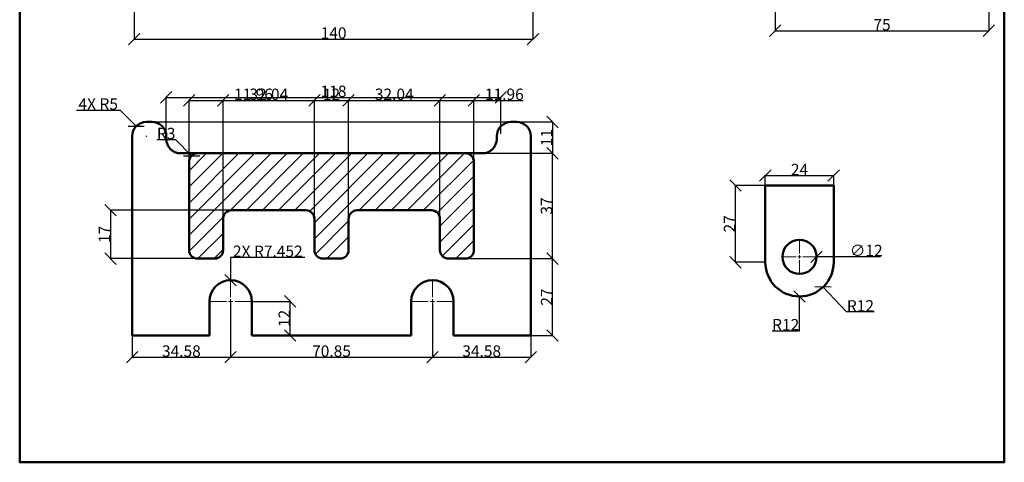
# Model space of a CAD drawing. Units: millimetres. Extents: x -13 to 343, y 323 to 787.
# Tile 1 of 3: x -13 to 333, y 323 to 479. Entities that reach past the tile are written whole.
import ezdxf

# ---------------------------------------------------------------- set-up
doc = ezdxf.new("R2010")
doc.units = ezdxf.units.MM
doc.header["$MEASUREMENT"] = 0
doc.header["$PDMODE"] = 3
doc.header["$PDSIZE"] = -8
doc.linetypes.add('CENTER', pattern=[50.8, 31.75, -6.35, 6.35, -6.35])
for name, color, linetype, lineweight in [('M-CNTR', 1, 'CENTER', 18), ('M-DIMS', 2, 'Continuous', 25), ('M-HATC', 8, 'Continuous', 18), ('M-OUTL', 7, 'Continuous', 50), ('M-TTLB', 7, 'Continuous', 50)]:
    doc.layers.add(name, color=color, linetype=linetype, lineweight=lineweight)
doc.styles.get("Standard").update_dxf_attribs({"font": 'arial.ttf'})
doc.dimstyles.get("Standard").update_dxf_attribs({"dimtxt": 4, "dimasz": 4, "dimexe": 0.18, "dimexo": 0.0625, "dimgap": 0.09, "dimtad": 1, "dimtoh": 1, "dimdec": 0, "dimzin": 0, "dimdsep": 46, "dimtxsty": 'Standard', "dimblk": 'OBLIQUE', "dimcen": 0.09, "dimclre": 251, "dimadec": 0, "dimazin": 0, "dimtfac": 1, "dimtdec": 0, "dimtofl": 0, "dimtmove": 0, "dimatfit": 3, "dimfxl": 1, "dimtolj": 1, "dimtzin": 0, "dimarcsym": 0})

# ---------------------------------------------------------------- blocks, each defined once
blk = doc.blocks.new('*U2')
at = {"layer": 'M-CNTR', "color": 0, "transparency": 16777216}
for p, q in [((0, 1.49), (0, 7.57)), ((-7.57, 0), (-1.49, 0)), ((1.49, 0), (7.57, 0)), ((0, -7.57), (0, -1.49))]:
    blk.add_line(p, q, dxfattribs=at)
at = {"layer": 'M-CNTR', "color": 0, "linetype": 'Continuous', "transparency": 16777216}
for p, q in [((-0.75, 0), (0.75, 0)), ((0, -0.75), (0, 0.75))]:
    blk.add_line(p, q, dxfattribs=at)
blk = doc.blocks.new('*U3')
at = {"layer": 'M-CNTR', "color": 0, "transparency": 16777216}
for p, q in [((0, 1.49), (0, 7.57)), ((-7.57, 0), (-1.49, 0)), ((1.49, 0), (7.57, 0)), ((0, -7.57), (0, -1.49))]:
    blk.add_line(p, q, dxfattribs=at)
at = {"layer": 'M-CNTR', "color": 0, "linetype": 'Continuous', "transparency": 16777216}
for p, q in [((-0.75, 0), (0.75, 0)), ((0, -0.75), (0, 0.75))]:
    blk.add_line(p, q, dxfattribs=at)
blk = doc.blocks.new('_Oblique')
at = {"color": 0, "linetype": 'ByBlock', "lineweight": -2}
blk.add_line((-0.5, -0.5), (0.5, 0.5), dxfattribs=at)
blk = doc.blocks.new('*D15')
at = {"layer": 'Defpoints', "color": 0, "transparency": 16777216}
for p in [(27.05, 495.9), (167.05, 495.9), (167.05, 471.86)]:
    blk.add_point(p, dxfattribs=at)
at = {"layer": 'M-DIMS', "color": 0, "lineweight": -2, "transparency": 16777216}
for p, q in [((27.05, 495.83), (27.05, 471.68)), ((167.05, 495.83), (167.05, 471.68)), ((27.05, 471.86), (167.05, 471.86))]:
    blk.add_line(p, q, dxfattribs=at)
at = {"layer": 'M-DIMS', "color": 0, "lineweight": -2, "transparency": 16777216, "xscale": 4, "yscale": 4, "zscale": 4, "rotation": 180}
blk.add_blockref('_Oblique', (27.05, 471.86), dxfattribs=at)
at = {"layer": 'M-DIMS', "color": 0, "lineweight": -2, "transparency": 16777216, "xscale": 4, "yscale": 4, "zscale": 4}
blk.add_blockref('_Oblique', (167.05, 471.86), dxfattribs=at)
at = {"layer": 'M-DIMS', "color": 0, "transparency": 16777216, "insert": (97.05, 473.99), "char_height": 4, "attachment_point": 5}
blk.add_mtext('\\A1;140', dxfattribs=at)
blk = doc.blocks.new('*D32')
at = {"layer": 'Defpoints', "color": 0, "transparency": 16777216}
for p in [(252.08, 495.9), (327.08, 495.9), (327.08, 474.82)]:
    blk.add_point(p, dxfattribs=at)
at = {"layer": 'M-DIMS', "color": 0, "lineweight": -2, "transparency": 16777216}
for p, q in [((252.08, 495.83), (252.08, 474.64)), ((327.08, 495.83), (327.08, 474.64)), ((252.08, 474.82), (327.08, 474.82))]:
    blk.add_line(p, q, dxfattribs=at)
at = {"layer": 'M-DIMS', "color": 0, "lineweight": -2, "transparency": 16777216, "xscale": 4, "yscale": 4, "zscale": 4, "rotation": 180}
blk.add_blockref('_Oblique', (252.08, 474.82), dxfattribs=at)
at = {"layer": 'M-DIMS', "color": 0, "lineweight": -2, "transparency": 16777216, "xscale": 4, "yscale": 4, "zscale": 4}
blk.add_blockref('_Oblique', (327.08, 474.82), dxfattribs=at)
at = {"layer": 'M-DIMS', "color": 0, "transparency": 16777216, "insert": (289.58, 476.94), "char_height": 4, "attachment_point": 5}
blk.add_mtext('\\A1;75', dxfattribs=at)
blk = doc.blocks.new('*D33')
at = {"layer": 'Defpoints', "color": 0, "transparency": 16777216}
for p in [(155.79, 451.41), (38.28, 438.48), (155.79, 438.48)]:
    blk.add_point(p, dxfattribs=at)
at = {"layer": 'M-DIMS', "color": 0, "lineweight": -2, "transparency": 16777216}
for p, q in [((38.28, 438.54), (38.28, 451.59)), ((38.28, 451.41), (155.79, 451.41)), ((155.79, 438.54), (155.79, 451.59))]:
    blk.add_line(p, q, dxfattribs=at)
at = {"layer": 'M-DIMS', "color": 0, "lineweight": -2, "transparency": 16777216, "xscale": 4, "yscale": 4, "zscale": 4, "rotation": 180}
blk.add_blockref('_Oblique', (38.28, 451.41), dxfattribs=at)
at = {"layer": 'M-DIMS', "color": 0, "lineweight": -2, "transparency": 16777216, "xscale": 4, "yscale": 4, "zscale": 4}
blk.add_blockref('_Oblique', (155.79, 451.41), dxfattribs=at)
at = {"layer": 'M-DIMS', "color": 0, "transparency": 16777216, "insert": (97.03, 453.54), "char_height": 4, "attachment_point": 5}
blk.add_mtext('\\A1;118', dxfattribs=at)
blk = doc.blocks.new('*D34')
at = {"layer": 'Defpoints', "color": 0, "transparency": 16777216}
for p in [(68.48, 379.75), (81.84, 379.75), (75.74, 367.75)]:
    blk.add_point(p, dxfattribs=at)
at = {"layer": 'M-DIMS', "color": 0, "lineweight": -2, "transparency": 16777216}
for p, q in [((68.54, 379.75), (82.02, 379.75)), ((81.84, 367.75), (81.84, 379.75)), ((75.8, 367.75), (82.02, 367.75))]:
    blk.add_line(p, q, dxfattribs=at)
at = {"layer": 'M-DIMS', "color": 0, "lineweight": -2, "transparency": 16777216, "xscale": 4, "yscale": 4, "zscale": 4}
for p, rotation in [((81.84, 379.75), 90), ((81.84, 367.75), 270)]:
    blk.add_blockref('_Oblique', p, dxfattribs=dict(at, rotation=rotation))
at = {"layer": 'M-DIMS', "color": 0, "transparency": 16777216, "insert": (79.74, 373.75), "char_height": 4, "attachment_point": 5, "rotation": 90}
blk.add_mtext('\\A1;12', dxfattribs=at)
blk = doc.blocks.new('*U35')
at = {"layer": 'M-CNTR', "color": 0, "transparency": 16777216}
for p, q in [((0, 1.2), (0, 6.12)), ((-6.12, 0), (-1.2, 0)), ((1.2, 0), (6.12, 0)), ((0, -6.12), (0, -1.2))]:
    blk.add_line(p, q, dxfattribs=at)
at = {"layer": 'M-CNTR', "color": 0, "linetype": 'Continuous', "transparency": 16777216}
for p, q in [((-0.6, 0), (0.6, 0)), ((0, -0.6), (0, 0.6))]:
    blk.add_line(p, q, dxfattribs=at)
blk = doc.blocks.new('*D36')
at = {"layer": 'Defpoints', "color": 0, "transparency": 16777216}
for p in [(238.13, 420.46), (248.61, 420.46), (248.61, 393.46)]:
    blk.add_point(p, dxfattribs=at)
at = {"layer": 'M-DIMS', "color": 0, "lineweight": -2, "transparency": 16777216}
for p, q in [((248.54, 420.46), (237.95, 420.46)), ((238.13, 393.46), (238.13, 420.46)), ((248.54, 393.46), (237.95, 393.46))]:
    blk.add_line(p, q, dxfattribs=at)
at = {"layer": 'M-DIMS', "color": 0, "lineweight": -2, "transparency": 16777216, "xscale": 4, "yscale": 4, "zscale": 4}
for p, rotation in [((238.13, 420.46), 90), ((238.13, 393.46), 270)]:
    blk.add_blockref('_Oblique', p, dxfattribs=dict(at, rotation=rotation))
at = {"layer": 'M-DIMS', "color": 0, "transparency": 16777216, "insert": (236.03, 406.96), "char_height": 4, "attachment_point": 5, "rotation": 90}
blk.add_mtext('\\A1;27', dxfattribs=at)
blk = doc.blocks.new('*D37')
at = {"layer": 'Defpoints', "color": 0, "transparency": 16777216}
for p in [(260.61, 393.46), (268.87, 384.77)]:
    blk.add_point(p, dxfattribs=at)
at = {"layer": 'M-DIMS', "color": 0, "lineweight": -2, "transparency": 16777216}
for p, q in [((260.52, 393.46), (260.7, 393.46)), ((260.61, 393.37), (260.61, 393.55)), ((277.15, 376.06), (268.87, 384.77)), ((286.76, 376.06), (277.15, 376.06))]:
    blk.add_line(p, q, dxfattribs=at)
at = {"layer": 'M-DIMS', "color": 0, "lineweight": -2, "transparency": 16777216, "xscale": 4, "yscale": 4, "zscale": 4, "rotation": 133.5491002898065}
blk.add_blockref('_Oblique', (268.87, 384.77), dxfattribs=at)
at = {"layer": 'M-DIMS', "color": 0, "transparency": 16777216, "insert": (282, 378.16), "char_height": 4, "attachment_point": 5}
blk.add_mtext('\\A1;R12', dxfattribs=at)
blk = doc.blocks.new('*D45')
at = {"layer": 'Defpoints', "color": 0, "transparency": 16777216}
for p in [(60.91, 379.75), (26.33, 367.75), (60.91, 360.15)]:
    blk.add_point(p, dxfattribs=at)
at = {"layer": 'M-DIMS', "color": 251, "lineweight": -2, "transparency": 16777216}
for p, q in [((60.91, 379.69), (60.91, 359.97)), ((26.33, 367.69), (26.33, 359.97))]:
    blk.add_line(p, q, dxfattribs=at)
at = {"layer": 'M-DIMS', "color": 0, "lineweight": -2, "transparency": 16777216}
blk.add_line((26.33, 360.15), (60.91, 360.15), dxfattribs=at)
at = {"layer": 'M-DIMS', "color": 0, "lineweight": -2, "transparency": 16777216, "xscale": 4, "yscale": 4, "zscale": 4, "rotation": 180}
blk.add_blockref('_Oblique', (26.33, 360.15), dxfattribs=at)
at = {"layer": 'M-DIMS', "color": 0, "lineweight": -2, "transparency": 16777216, "xscale": 4, "yscale": 4, "zscale": 4}
blk.add_blockref('_Oblique', (60.91, 360.15), dxfattribs=at)
at = {"layer": 'M-DIMS', "color": 0, "transparency": 16777216, "insert": (43.62, 362.28), "char_height": 4, "attachment_point": 5}
blk.add_mtext('\\A1;34.58', dxfattribs=at)
blk = doc.blocks.new('*D46')
at = {"layer": 'Defpoints', "color": 0, "transparency": 16777216}
for p in [(60.91, 379.75), (131.75, 379.75), (131.75, 360.15)]:
    blk.add_point(p, dxfattribs=at)
at = {"layer": 'M-DIMS', "color": 251, "lineweight": -2, "transparency": 16777216}
for p, q in [((60.91, 379.69), (60.91, 359.97)), ((131.75, 379.69), (131.75, 359.97))]:
    blk.add_line(p, q, dxfattribs=at)
at = {"layer": 'M-DIMS', "color": 0, "lineweight": -2, "transparency": 16777216}
blk.add_line((60.91, 360.15), (131.75, 360.15), dxfattribs=at)
at = {"layer": 'M-DIMS', "color": 0, "lineweight": -2, "transparency": 16777216, "xscale": 4, "yscale": 4, "zscale": 4, "rotation": 180}
blk.add_blockref('_Oblique', (60.91, 360.15), dxfattribs=at)
at = {"layer": 'M-DIMS', "color": 0, "lineweight": -2, "transparency": 16777216, "xscale": 4, "yscale": 4, "zscale": 4}
blk.add_blockref('_Oblique', (131.75, 360.15), dxfattribs=at)
at = {"layer": 'M-DIMS', "color": 0, "transparency": 16777216, "insert": (96.33, 362.28), "char_height": 4, "attachment_point": 5}
blk.add_mtext('\\A1;70.85', dxfattribs=at)
blk = doc.blocks.new('*D47')
at = {"layer": 'Defpoints', "color": 0, "transparency": 16777216}
for p in [(131.75, 379.75), (166.33, 367.75), (166.33, 360.15)]:
    blk.add_point(p, dxfattribs=at)
at = {"layer": 'M-DIMS', "color": 251, "lineweight": -2, "transparency": 16777216}
for p, q in [((131.75, 379.69), (131.75, 359.97)), ((166.33, 367.69), (166.33, 359.97))]:
    blk.add_line(p, q, dxfattribs=at)
at = {"layer": 'M-DIMS', "color": 0, "lineweight": -2, "transparency": 16777216}
blk.add_line((131.75, 360.15), (166.33, 360.15), dxfattribs=at)
at = {"layer": 'M-DIMS', "color": 0, "lineweight": -2, "transparency": 16777216, "xscale": 4, "yscale": 4, "zscale": 4, "rotation": 180}
blk.add_blockref('_Oblique', (131.75, 360.15), dxfattribs=at)
at = {"layer": 'M-DIMS', "color": 0, "lineweight": -2, "transparency": 16777216, "xscale": 4, "yscale": 4, "zscale": 4}
blk.add_blockref('_Oblique', (166.33, 360.15), dxfattribs=at)
at = {"layer": 'M-DIMS', "color": 0, "transparency": 16777216, "insert": (149.04, 362.28), "char_height": 4, "attachment_point": 5}
blk.add_mtext('\\A1;34.58', dxfattribs=at)
blk = doc.blocks.new('*D48')
at = {"layer": 'Defpoints', "color": 0, "transparency": 16777216}
for p in [(33.33, 442.75), (43.33, 431.75), (173.93, 431.75)]:
    blk.add_point(p, dxfattribs=at)
at = {"layer": 'M-DIMS', "color": 251, "lineweight": -2, "transparency": 16777216}
for p, q in [((33.39, 442.75), (174.11, 442.75)), ((43.39, 431.75), (174.11, 431.75))]:
    blk.add_line(p, q, dxfattribs=at)
at = {"layer": 'M-DIMS', "color": 0, "lineweight": -2, "transparency": 16777216}
blk.add_line((173.93, 442.75), (173.93, 431.75), dxfattribs=at)
at = {"layer": 'M-DIMS', "color": 0, "lineweight": -2, "transparency": 16777216, "xscale": 4, "yscale": 4, "zscale": 4}
for p, rotation in [((173.93, 442.75), 90), ((173.93, 431.75), 270)]:
    blk.add_blockref('_Oblique', p, dxfattribs=dict(at, rotation=rotation))
at = {"layer": 'M-DIMS', "color": 0, "transparency": 16777216, "insert": (171.83, 437.25), "char_height": 4, "attachment_point": 5, "rotation": 90}
blk.add_mtext('\\A1;11', dxfattribs=at)
blk = doc.blocks.new('*D49')
at = {"layer": 'Defpoints', "color": 0, "transparency": 16777216}
for p in [(143.33, 394.75), (173.93, 394.75), (166.33, 367.75)]:
    blk.add_point(p, dxfattribs=at)
at = {"layer": 'M-DIMS', "color": 251, "lineweight": -2, "transparency": 16777216}
for p, q in [((143.39, 394.75), (174.11, 394.75)), ((166.39, 367.75), (174.11, 367.75))]:
    blk.add_line(p, q, dxfattribs=at)
at = {"layer": 'M-DIMS', "color": 0, "lineweight": -2, "transparency": 16777216}
blk.add_line((173.93, 367.75), (173.93, 394.75), dxfattribs=at)
at = {"layer": 'M-DIMS', "color": 0, "lineweight": -2, "transparency": 16777216, "xscale": 4, "yscale": 4, "zscale": 4}
for p, rotation in [((173.93, 394.75), 90), ((173.93, 367.75), 270)]:
    blk.add_blockref('_Oblique', p, dxfattribs=dict(at, rotation=rotation))
at = {"layer": 'M-DIMS', "color": 0, "transparency": 16777216, "insert": (171.83, 381.25), "char_height": 4, "attachment_point": 5, "rotation": 90}
blk.add_mtext('\\A1;27', dxfattribs=at)
blk = doc.blocks.new('*D50')
at = {"layer": 'Defpoints', "color": 0, "transparency": 16777216}
for p in [(143.33, 431.75), (173.93, 431.75), (143.33, 394.75)]:
    blk.add_point(p, dxfattribs=at)
at = {"layer": 'M-DIMS', "color": 251, "lineweight": -2, "transparency": 16777216}
for p, q in [((143.39, 431.75), (174.11, 431.75)), ((143.39, 394.75), (174.11, 394.75))]:
    blk.add_line(p, q, dxfattribs=at)
at = {"layer": 'M-DIMS', "color": 0, "lineweight": -2, "transparency": 16777216}
blk.add_line((173.93, 394.75), (173.93, 431.75), dxfattribs=at)
at = {"layer": 'M-DIMS', "color": 0, "lineweight": -2, "transparency": 16777216, "xscale": 4, "yscale": 4, "zscale": 4}
for p, rotation in [((173.93, 431.75), 90), ((173.93, 394.75), 270)]:
    blk.add_blockref('_Oblique', p, dxfattribs=dict(at, rotation=rotation))
at = {"layer": 'M-DIMS', "color": 0, "transparency": 16777216, "insert": (171.79, 413.25), "char_height": 4, "attachment_point": 5, "rotation": 90}
blk.add_mtext('\\A1;37', dxfattribs=at)
blk = doc.blocks.new('*D51')
at = {"layer": 'Defpoints', "color": 0, "transparency": 16777216}
for p in [(58.29, 450.35), (46.33, 397.75), (58.29, 397.75)]:
    blk.add_point(p, dxfattribs=at)
at = {"layer": 'M-DIMS', "color": 251, "lineweight": -2, "transparency": 16777216}
for p, q in [((46.33, 397.81), (46.33, 450.53)), ((58.29, 397.81), (58.29, 450.53))]:
    blk.add_line(p, q, dxfattribs=at)
at = {"layer": 'M-DIMS', "color": 0, "lineweight": -2, "transparency": 16777216}
for p, q in [((46.33, 450.35), (58.29, 450.35)), ((58.29, 450.35), (75.59, 450.35))]:
    blk.add_line(p, q, dxfattribs=at)
at = {"layer": 'M-DIMS', "color": 0, "lineweight": -2, "transparency": 16777216, "xscale": 4, "yscale": 4, "zscale": 4, "rotation": 180}
blk.add_blockref('_Oblique', (46.33, 450.35), dxfattribs=at)
at = {"layer": 'M-DIMS', "color": 0, "lineweight": -2, "transparency": 16777216, "xscale": 4, "yscale": 4, "zscale": 4}
blk.add_blockref('_Oblique', (58.29, 450.35), dxfattribs=at)
at = {"layer": 'M-DIMS', "color": 0, "transparency": 16777216, "insert": (68.94, 452.48), "char_height": 4, "attachment_point": 5}
blk.add_mtext('\\A1;11.96', dxfattribs=at)
blk = doc.blocks.new('*D52')
at = {"layer": 'Defpoints', "color": 0, "transparency": 16777216}
for p in [(90.33, 450.35), (58.29, 397.75), (90.33, 397.75)]:
    blk.add_point(p, dxfattribs=at)
at = {"layer": 'M-DIMS', "color": 251, "lineweight": -2, "transparency": 16777216}
for p, q in [((58.29, 397.81), (58.29, 450.53)), ((90.33, 397.81), (90.33, 450.53))]:
    blk.add_line(p, q, dxfattribs=at)
at = {"layer": 'M-DIMS', "color": 0, "lineweight": -2, "transparency": 16777216}
blk.add_line((58.29, 450.35), (90.33, 450.35), dxfattribs=at)
at = {"layer": 'M-DIMS', "color": 0, "lineweight": -2, "transparency": 16777216, "xscale": 4, "yscale": 4, "zscale": 4, "rotation": 180}
blk.add_blockref('_Oblique', (58.29, 450.35), dxfattribs=at)
at = {"layer": 'M-DIMS', "color": 0, "lineweight": -2, "transparency": 16777216, "xscale": 4, "yscale": 4, "zscale": 4}
blk.add_blockref('_Oblique', (90.33, 450.35), dxfattribs=at)
at = {"layer": 'M-DIMS', "color": 0, "transparency": 16777216, "insert": (74.31, 452.48), "char_height": 4, "attachment_point": 5}
blk.add_mtext('\\A1;32.04', dxfattribs=at)
blk = doc.blocks.new('*D53')
at = {"layer": 'Defpoints', "color": 0, "transparency": 16777216}
for p in [(102.33, 450.35), (90.33, 397.75), (102.33, 397.75)]:
    blk.add_point(p, dxfattribs=at)
at = {"layer": 'M-DIMS', "color": 251, "lineweight": -2, "transparency": 16777216}
for p, q in [((90.33, 397.81), (90.33, 450.53)), ((102.33, 397.81), (102.33, 450.53))]:
    blk.add_line(p, q, dxfattribs=at)
at = {"layer": 'M-DIMS', "color": 0, "lineweight": -2, "transparency": 16777216}
blk.add_line((90.33, 450.35), (102.33, 450.35), dxfattribs=at)
at = {"layer": 'M-DIMS', "color": 0, "lineweight": -2, "transparency": 16777216, "xscale": 4, "yscale": 4, "zscale": 4, "rotation": 180}
blk.add_blockref('_Oblique', (90.33, 450.35), dxfattribs=at)
at = {"layer": 'M-DIMS', "color": 0, "lineweight": -2, "transparency": 16777216, "xscale": 4, "yscale": 4, "zscale": 4}
blk.add_blockref('_Oblique', (102.33, 450.35), dxfattribs=at)
at = {"layer": 'M-DIMS', "color": 0, "transparency": 16777216, "insert": (96.33, 452.45), "char_height": 4, "attachment_point": 5}
blk.add_mtext('\\A1;12', dxfattribs=at)
blk = doc.blocks.new('*D54')
at = {"layer": 'Defpoints', "color": 0, "transparency": 16777216}
for p in [(134.37, 450.35), (102.33, 397.75), (134.37, 397.75)]:
    blk.add_point(p, dxfattribs=at)
at = {"layer": 'M-DIMS', "color": 251, "lineweight": -2, "transparency": 16777216}
for p, q in [((102.33, 397.81), (102.33, 450.53)), ((134.37, 397.81), (134.37, 450.53))]:
    blk.add_line(p, q, dxfattribs=at)
at = {"layer": 'M-DIMS', "color": 0, "lineweight": -2, "transparency": 16777216}
blk.add_line((102.33, 450.35), (134.37, 450.35), dxfattribs=at)
at = {"layer": 'M-DIMS', "color": 0, "lineweight": -2, "transparency": 16777216, "xscale": 4, "yscale": 4, "zscale": 4, "rotation": 180}
blk.add_blockref('_Oblique', (102.33, 450.35), dxfattribs=at)
at = {"layer": 'M-DIMS', "color": 0, "lineweight": -2, "transparency": 16777216, "xscale": 4, "yscale": 4, "zscale": 4}
blk.add_blockref('_Oblique', (134.37, 450.35), dxfattribs=at)
at = {"layer": 'M-DIMS', "color": 0, "transparency": 16777216, "insert": (118.35, 452.48), "char_height": 4, "attachment_point": 5}
blk.add_mtext('\\A1;32.04', dxfattribs=at)
blk = doc.blocks.new('*D55')
at = {"layer": 'Defpoints', "color": 0, "transparency": 16777216}
for p in [(146.33, 450.35), (134.37, 397.75), (146.33, 397.75)]:
    blk.add_point(p, dxfattribs=at)
at = {"layer": 'M-DIMS', "color": 251, "lineweight": -2, "transparency": 16777216}
for p, q in [((134.37, 397.81), (134.37, 450.53)), ((146.33, 397.81), (146.33, 450.53))]:
    blk.add_line(p, q, dxfattribs=at)
at = {"layer": 'M-DIMS', "color": 0, "lineweight": -2, "transparency": 16777216}
for p, q in [((134.37, 450.35), (146.33, 450.35)), ((146.33, 450.35), (163.63, 450.35))]:
    blk.add_line(p, q, dxfattribs=at)
at = {"layer": 'M-DIMS', "color": 0, "lineweight": -2, "transparency": 16777216, "xscale": 4, "yscale": 4, "zscale": 4, "rotation": 180}
blk.add_blockref('_Oblique', (134.37, 450.35), dxfattribs=at)
at = {"layer": 'M-DIMS', "color": 0, "lineweight": -2, "transparency": 16777216, "xscale": 4, "yscale": 4, "zscale": 4}
blk.add_blockref('_Oblique', (146.33, 450.35), dxfattribs=at)
at = {"layer": 'M-DIMS', "color": 0, "transparency": 16777216, "insert": (156.98, 452.48), "char_height": 4, "attachment_point": 5}
blk.add_mtext('\\A1;11.96', dxfattribs=at)
blk = doc.blocks.new('*D56')
at = {"layer": 'Defpoints', "color": 0, "transparency": 16777216}
for p in [(61.29, 411.75), (18.73, 394.75), (49.33, 394.75)]:
    blk.add_point(p, dxfattribs=at)
at = {"layer": 'M-DIMS', "color": 251, "lineweight": -2, "transparency": 16777216}
for p, q in [((61.23, 411.75), (18.55, 411.75)), ((49.27, 394.75), (18.55, 394.75))]:
    blk.add_line(p, q, dxfattribs=at)
at = {"layer": 'M-DIMS', "color": 0, "lineweight": -2, "transparency": 16777216}
blk.add_line((18.73, 411.75), (18.73, 394.75), dxfattribs=at)
at = {"layer": 'M-DIMS', "color": 0, "lineweight": -2, "transparency": 16777216, "xscale": 4, "yscale": 4, "zscale": 4}
for p, rotation in [((18.73, 411.75), 90), ((18.73, 394.75), 270)]:
    blk.add_blockref('_Oblique', p, dxfattribs=dict(at, rotation=rotation))
at = {"layer": 'M-DIMS', "color": 0, "transparency": 16777216, "insert": (16.63, 403.25), "char_height": 4, "attachment_point": 5, "rotation": 90}
blk.add_mtext('\\A1;17', dxfattribs=at)
blk = doc.blocks.new('*D64')
at = {"layer": 'Defpoints', "color": 0, "transparency": 16777216}
for p in [(272.61, 423.96), (248.61, 420.46), (272.61, 420.46)]:
    blk.add_point(p, dxfattribs=at)
at = {"layer": 'M-DIMS', "color": 251, "lineweight": -2, "transparency": 16777216}
for p, q in [((248.61, 420.53), (248.61, 424.14)), ((272.61, 420.53), (272.61, 424.14))]:
    blk.add_line(p, q, dxfattribs=at)
at = {"layer": 'M-DIMS', "color": 0, "lineweight": -2, "transparency": 16777216}
blk.add_line((248.61, 423.96), (272.61, 423.96), dxfattribs=at)
at = {"layer": 'M-DIMS', "color": 0, "lineweight": -2, "transparency": 16777216, "xscale": 4, "yscale": 4, "zscale": 4, "rotation": 180}
blk.add_blockref('_Oblique', (248.61, 423.96), dxfattribs=at)
at = {"layer": 'M-DIMS', "color": 0, "lineweight": -2, "transparency": 16777216, "xscale": 4, "yscale": 4, "zscale": 4}
blk.add_blockref('_Oblique', (272.61, 423.96), dxfattribs=at)
at = {"layer": 'M-DIMS', "color": 0, "transparency": 16777216, "insert": (260.61, 426.06), "char_height": 4, "attachment_point": 5}
blk.add_mtext('\\A1;24', dxfattribs=at)
blk = doc.blocks.new('*D71')
at = {"layer": 'Defpoints', "color": 0, "transparency": 16777216}
for p in [(60.91, 387.2), (60.91, 379.75)]:
    blk.add_point(p, dxfattribs=at)
at = {"layer": 'M-DIMS', "color": 0, "lineweight": -2, "transparency": 16777216}
for p, q in [((86.94, 395.2), (60.91, 395.2)), ((60.91, 395.2), (60.91, 387.2))]:
    blk.add_line(p, q, dxfattribs=at)
at = {"layer": 'M-DIMS', "color": 251, "lineweight": -2, "transparency": 16777216}
for p, q in [((60.82, 379.75), (61, 379.75)), ((60.91, 379.66), (60.91, 379.84))]:
    blk.add_line(p, q, dxfattribs=at)
at = {"layer": 'M-DIMS', "color": 0, "lineweight": -2, "transparency": 16777216, "xscale": 4, "yscale": 4, "zscale": 4, "rotation": 269.9962400545088}
blk.add_blockref('_Oblique', (60.91, 387.2), dxfattribs=at)
at = {"layer": 'M-DIMS', "color": 0, "transparency": 16777216, "insert": (73.97, 397.33), "char_height": 4, "attachment_point": 5}
blk.add_mtext('\\A1;2X R7.452', dxfattribs=at)
blk = doc.blocks.new('*D72')
at = {"layer": 'Defpoints', "color": 0, "transparency": 16777216}
for p in [(27.79, 441.29), (31.33, 437.75)]:
    blk.add_point(p, dxfattribs=at)
at = {"layer": 'M-DIMS', "color": 0, "lineweight": -2, "transparency": 16777216}
for p, q in [((6.81, 446.94), (22.14, 446.94)), ((22.14, 446.94), (27.79, 441.29))]:
    blk.add_line(p, q, dxfattribs=at)
at = {"layer": 'M-DIMS', "color": 251, "lineweight": -2, "transparency": 16777216}
for p, q in [((31.24, 437.75), (31.42, 437.75)), ((31.33, 437.66), (31.33, 437.84))]:
    blk.add_line(p, q, dxfattribs=at)
at = {"layer": 'M-DIMS', "color": 0, "lineweight": -2, "transparency": 16777216, "xscale": 4, "yscale": 4, "zscale": 4, "rotation": 314.9991735096431}
blk.add_blockref('_Oblique', (27.79, 441.29), dxfattribs=at)
at = {"layer": 'M-DIMS', "color": 0, "transparency": 16777216, "insert": (14.43, 449.07), "char_height": 4, "attachment_point": 5}
blk.add_mtext('\\A1;4X R5', dxfattribs=at)
blk = doc.blocks.new('*D73')
at = {"layer": 'Defpoints', "color": 0, "transparency": 16777216}
for p in [(47.22, 430.88), (49.33, 428.75)]:
    blk.add_point(p, dxfattribs=at)
at = {"layer": 'M-DIMS', "color": 0, "lineweight": -2, "transparency": 16777216}
for p, q in [((35.05, 436.57), (41.59, 436.57)), ((41.59, 436.57), (47.22, 430.88))]:
    blk.add_line(p, q, dxfattribs=at)
at = {"layer": 'M-DIMS', "color": 251, "lineweight": -2, "transparency": 16777216}
for p, q in [((49.24, 428.75), (49.42, 428.75)), ((49.33, 428.66), (49.33, 428.84))]:
    blk.add_line(p, q, dxfattribs=at)
at = {"layer": 'M-DIMS', "color": 0, "lineweight": -2, "transparency": 16777216, "xscale": 4, "yscale": 4, "zscale": 4, "rotation": 314.7064054961642}
blk.add_blockref('_Oblique', (47.22, 430.88), dxfattribs=at)
at = {"layer": 'M-DIMS', "color": 0, "transparency": 16777216, "insert": (38.28, 438.7), "char_height": 4, "attachment_point": 5}
blk.add_mtext('\\A1;R3', dxfattribs=at)
blk = doc.blocks.new('*D78')
at = {"layer": 'Defpoints', "color": 0, "transparency": 16777216}
for p in [(260.61, 393.46), (260.61, 381.46)]:
    blk.add_point(p, dxfattribs=at)
at = {"layer": 'M-DIMS', "color": 251, "lineweight": -2, "transparency": 16777216}
for p, q in [((260.52, 393.46), (260.7, 393.46)), ((260.61, 393.37), (260.61, 393.55))]:
    blk.add_line(p, q, dxfattribs=at)
at = {"layer": 'M-DIMS', "color": 0, "lineweight": -2, "transparency": 16777216}
for p, q in [((260.61, 369.45), (260.61, 381.46)), ((251, 369.45), (260.61, 369.45))]:
    blk.add_line(p, q, dxfattribs=at)
at = {"layer": 'M-DIMS', "color": 0, "lineweight": -2, "transparency": 16777216, "xscale": 4, "yscale": 4, "zscale": 4, "rotation": 89.99963712672984}
blk.add_blockref('_Oblique', (260.61, 381.46), dxfattribs=at)
at = {"layer": 'M-DIMS', "color": 0, "transparency": 16777216, "insert": (255.76, 371.55), "char_height": 4, "attachment_point": 5}
blk.add_mtext('\\A1;R12', dxfattribs=at)
blk = doc.blocks.new('*D79')
at = {"layer": 'Defpoints', "color": 0, "transparency": 16777216}
for p in [(254.61, 395.38), (266.61, 395.38)]:
    blk.add_point(p, dxfattribs=at)
at = {"layer": 'M-DIMS', "color": 251, "lineweight": -2, "transparency": 16777216}
for p, q in [((260.52, 395.38), (260.7, 395.38)), ((260.61, 395.29), (260.61, 395.47))]:
    blk.add_line(p, q, dxfattribs=at)
at = {"layer": 'M-DIMS', "color": 0, "lineweight": -2, "transparency": 16777216}
for p, q in [((278.92, 395.38), (266.61, 395.38)), ((289.05, 395.38), (278.92, 395.38))]:
    blk.add_line(p, q, dxfattribs=at)
at = {"layer": 'M-DIMS', "color": 0, "lineweight": -2, "transparency": 16777216, "xscale": 4, "yscale": 4, "zscale": 4, "rotation": 179.99955118306}
blk.add_blockref('_Oblique', (266.61, 395.38), dxfattribs=at)
at = {"layer": 'M-DIMS', "color": 0, "transparency": 16777216, "insert": (284.03, 397.62), "char_height": 4, "attachment_point": 5}
blk.add_mtext('\\A1;∅12', dxfattribs=at)

msp = doc.modelspace()

# ---------------------------------------------------------------- hatches: boundary and pattern name
at = {"layer": 'M-HATC'}
h = msp.add_hatch(dxfattribs=at)
h.set_pattern_fill('ANSI31', color=256, scale=32)
h.set_pattern_definition([(45, (-0.7245, -0.4755), (-2.828427, 2.828427), [])])
h.paths.add_polyline_path([(90.3284, 408.7504), (90.3284, 397.7504, 0.41421356), (93.3284, 394.7504), (99.3284, 394.7504, 0.41421356), (102.3284, 397.7504), (102.3284, 408.7504, -0.41421356), (105.3284, 411.7504), (131.3675, 411.7504, -0.41421356), (134.3675, 408.7504), (134.3675, 397.7504, 0.41421356), (137.3675, 394.7504), (143.3284, 394.7504, 0.41421356), (146.3284, 397.7504), (146.3284, 428.7504, 0.41421356), (143.3284, 431.7504), (49.3284, 431.7504, 0.41421356), (46.3284, 428.7504), (46.3284, 397.7504, 0.41421356), (49.3284, 394.7504), (55.2894, 394.7504, 0.41421356), (58.2894, 397.7504), (58.2894, 408.7504, -0.41421356), (61.2894, 411.7504), (87.3284, 411.7504, -0.41421356)])

# ---------------------------------------------------------------- linework, layer by layer
at = {"layer": 'M-OUTL'}
for p, q in [((31.3284, 442.7504), (33.3284, 442.7504)), ((159.3284, 442.7504), (161.3284, 442.7504)), ((26.3284, 437.7504), (26.3284, 367.7504)), ((38.3284, 436.7504), (38.3284, 437.7504)), ((154.3284, 437.7504), (154.3284, 436.7504)), ((166.3284, 437.7504), (166.3284, 367.7504)), ((43.3284, 431.7504), (149.3284, 431.7504)), ((46.3284, 397.7504), (46.3284, 428.7504)), ((146.3284, 428.7504), (146.3284, 397.7504)), ((248.6071, 393.4648), (248.6071, 420.4648)), ((248.6071, 420.4648), (272.6071, 420.4648)), ((272.6071, 393.4648), (272.6071, 420.4648)), ((61.2894, 411.7504), (87.3284, 411.7504)), ((105.3284, 411.7504), (131.3675, 411.7504)), ((58.2894, 408.7504), (58.2894, 397.7504)), ((90.3284, 397.7504), (90.3284, 408.7504)), ((102.3284, 397.7504), (102.3284, 408.7504)), ((134.3675, 408.7504), (134.3675, 397.7504)), ((49.3284, 394.7504), (55.2894, 394.7504)), ((93.3284, 394.7504), (99.3284, 394.7504)), ((137.3675, 394.7504), (143.3284, 394.7504)), ((53.4539, 379.7504), (53.4539, 367.7504)), ((68.3571, 379.7504), (68.3571, 367.7504)), ((124.2998, 379.7504), (124.2998, 367.7504)), ((139.203, 379.7504), (139.203, 367.7504)), ((26.3284, 367.7504), (53.4539, 367.7504)), ((68.3571, 367.7504), (124.2998, 367.7504)), ((139.203, 367.7504), (166.3284, 367.7504))]:
    msp.add_line(p, q, dxfattribs=at)
msp.add_circle((260.6071, 395.376), 6, dxfattribs=at)
for centre, radius, start, end in [((31.3284, 437.7504), 5, 90, 180), ((33.3284, 437.7504), 5, 0, 90), ((159.3284, 437.7504), 5, 90, 180), ((161.3284, 437.7504), 5, 360, 90), ((43.3284, 436.7504), 5, 180, 270), ((149.3284, 436.7504), 5, 270, 0), ((49.3284, 428.7504), 3, 90, 180), ((143.3284, 428.7504), 3, 0, 90), ((61.2894, 408.7504), 3, 90, 180), ((87.3284, 408.7504), 3, 0, 90), ((105.3284, 408.7504), 3, 90, 180), ((131.3675, 408.7504), 3, 0, 90), ((49.3284, 397.7504), 3, 180, 270), ((55.2894, 397.7504), 3, 270, 0), ((93.3284, 397.7504), 3, 180, 270), ((99.3284, 397.7504), 3, 270, 0), ((137.3675, 397.7504), 3, 180, 270), ((143.3284, 397.7504), 3, 270, 0), ((260.6071, 393.4648), 12, 180, 0), ((60.9055, 379.7504), 7.4516, 0, 180), ((131.7514, 379.7504), 7.4516, 0, 180)]:
    msp.add_arc(centre, radius, start, end, dxfattribs=at)
at = {"layer": 'M-TTLB'}
msp.add_lwpolyline([(-13.1348, 787.3025), (332.5007, 787.3025), (332.5007, 323.2082), (-13.1348, 323.2082)], close=True, dxfattribs=at)

# ---------------------------------------------------------------- block references
at = {"layer": 'M-CNTR'}
for name, p in [('*U35', (260.6071, 395.376)), ('*U2', (60.9055, 379.7504)), ('*U3', (131.7514, 379.7504))]:
    msp.add_blockref(name, p, dxfattribs=at)

# ---------------------------------------------------------------- dimensions: what is measured, and where the dimension line sits
at = {"layer": 'M-DIMS'}
for base, p1, p2, override, picture, middle in [((167.053, 471.8556), (27.053, 495.8961), (167.053, 495.8961), {"dimclrd": 0, "dimclre": 0, "dimclrt": 0}, '*D15', (97.053, 473.9879)), ((327.0764, 474.8184), (252.0764, 495.8961), (327.0764, 495.8961), {"dimclrd": 0, "dimclre": 0, "dimclrt": 0}, '*D32', (289.5764, 476.9425)), ((155.7929, 451.4061), (38.2756, 438.4752), (155.7929, 438.4752), {"dimclrd": 0, "dimclre": 0, "dimclrt": 0}, '*D33', (97.0343, 453.5384)), ((58.2894, 450.3504), (46.3284, 397.7504), (58.2894, 397.7504), {"dimdec": 2, "dimlfac": 1, "dimrnd": 0, "dimzin": 0, "dimdsep": 46, "dimlunit": 2}, '*D51', (68.9388, 452.4827)), ((90.3284, 450.3504), (58.2894, 397.7504), (90.3284, 397.7504), {"dimdec": 2, "dimlfac": 1, "dimrnd": 0, "dimzin": 0, "dimdsep": 46, "dimlunit": 2}, '*D52', (74.3089, 452.4841)), ((102.3284, 450.3504), (90.3284, 397.7504), (102.3284, 397.7504), {"dimdec": 0, "dimlfac": 1, "dimrnd": 0, "dimzin": 0, "dimdsep": 46, "dimlunit": 2}, '*D53', (96.3284, 452.4486)), ((134.3675, 450.3504), (102.3284, 397.7504), (134.3675, 397.7504), {"dimdec": 2, "dimlfac": 1, "dimrnd": 0, "dimzin": 0, "dimdsep": 46, "dimlunit": 2}, '*D54', (118.348, 452.4841)), ((146.3284, 450.3504), (134.3675, 397.7504), (146.3284, 397.7504), {"dimdec": 2, "dimlfac": 1, "dimrnd": 0, "dimzin": 0, "dimdsep": 46, "dimlunit": 2}, '*D55', (156.9778, 452.4827)), ((272.6071, 423.9648), (248.6071, 420.4648), (272.6071, 420.4648), {"dimdec": 0, "dimlfac": 1, "dimrnd": 0, "dimzin": 0, "dimdsep": 46, "dimlunit": 2}, '*D64', (260.6071, 426.063)), ((60.9055, 360.1504), (26.3284, 367.7504), (60.9055, 379.7504), {"dimdec": 2, "dimlfac": 1, "dimrnd": 0, "dimzin": 0, "dimdsep": 46, "dimlunit": 2}, '*D45', (43.617, 362.2841)), ((131.7514, 360.1504), (60.9055, 379.7504), (131.7514, 379.7504), {"dimdec": 2, "dimlfac": 1, "dimrnd": 0, "dimzin": 0, "dimdsep": 46, "dimlunit": 2}, '*D46', (96.3284, 362.2827)), ((166.3284, 360.1504), (131.7514, 379.7504), (166.3284, 367.7504), {"dimdec": 2, "dimlfac": 1, "dimrnd": 0, "dimzin": 0, "dimdsep": 46, "dimlunit": 2}, '*D47', (149.0399, 362.2841))]:
    dim = msp.add_linear_dim(base=base, p1=p1, p2=p2, dimstyle='Standard', override=override, dxfattribs=at)
    dim.commit()
    dim.dimension.update_dxf_attribs({"geometry": picture, "text_midpoint": middle})
for center, mpoint, text, override, picture, middle in [((31.3284, 437.7504), (27.793, 441.286), '4X <>', {"dimdec": 0, "dimlfac": 1, "dimrnd": 0, "dimzin": 0, "dimdsep": 46, "dimlunit": 2}, '*D72', (14.4282, 449.0671)), ((60.9055, 379.7504), (60.906, 387.2021), '2X <>', {"dimdec": 3, "dimlfac": 1, "dimrnd": 0, "dimzin": 0, "dimdsep": 46, "dimlunit": 2}, '*D71', (73.9706, 397.3343))]:
    dim = msp.add_radius_dim(center=center, mpoint=mpoint, text=text, dimstyle='Standard', override=override, dxfattribs=at)
    dim.commit()
    dim.dimension.update_dxf_attribs({"geometry": picture, "text_midpoint": middle})
for base, p1, p2, override, picture, middle in [((173.9284, 431.7504), (33.3284, 442.7504), (43.3284, 431.7504), {"dimdec": 0, "dimlfac": 1, "dimrnd": 0, "dimzin": 0, "dimdsep": 46, "dimlunit": 2}, '*D48', (171.8303, 437.2504)), ((173.9284, 431.7504), (143.3284, 394.7504), (143.3284, 431.7504), {"dimdec": 0, "dimlfac": 1, "dimrnd": 0, "dimzin": 0, "dimdsep": 46, "dimlunit": 2}, '*D50', (171.7948, 413.2504)), ((238.1317, 420.4648), (248.6071, 393.4648), (248.6071, 420.4648), {"dimclrd": 0, "dimclre": 0, "dimclrt": 0}, '*D36', (236.0335, 406.9648)), ((18.7284, 394.7504), (61.2894, 411.7504), (49.3284, 394.7504), {"dimdec": 0, "dimlfac": 1, "dimrnd": 0, "dimzin": 0, "dimdsep": 46, "dimlunit": 2}, '*D56', (16.6303, 403.2504)), ((173.9284, 394.7504), (166.3284, 367.7504), (143.3284, 394.7504), {"dimdec": 0, "dimlfac": 1, "dimrnd": 0, "dimzin": 0, "dimdsep": 46, "dimlunit": 2}, '*D49', (171.8303, 381.2504)), ((81.8357, 379.7504), (75.7408, 367.7504), (68.4771, 379.7504), {"dimclrd": 0, "dimclre": 0, "dimclrt": 0}, '*D34', (79.7375, 373.7504))]:
    dim = msp.add_linear_dim(base=base, p1=p1, p2=p2, angle=90, dimstyle='Standard', override=override, dxfattribs=at)
    dim.commit()
    dim.dimension.update_dxf_attribs({"geometry": picture, "text_midpoint": middle})
for center, mpoint, override, picture, middle in [((49.3284, 428.7504), (47.218, 430.8826), {"dimdec": 0, "dimlfac": 1, "dimrnd": 0, "dimzin": 0, "dimdsep": 46, "dimlunit": 2}, '*D73', (38.2751, 438.702)), ((260.6071, 393.4648), (260.607, 381.4648), {"dimdec": 0, "dimlfac": 1, "dimrnd": 0, "dimzin": 0, "dimdsep": 46, "dimlunit": 2}, '*D78', (255.7584, 371.5466)), ((260.6071, 393.4648), (268.8748, 384.7674), {"dimclrd": 0, "dimclre": 0, "dimclrt": 0}, '*D37', (282.0023, 378.1563))]:
    dim = msp.add_radius_dim(center=center, mpoint=mpoint, dimstyle='Standard', override=override, dxfattribs=at)
    dim.commit()
    dim.dimension.update_dxf_attribs({"geometry": picture, "text_midpoint": middle})
dim = msp.add_diameter_dim_2p(p1=(254.6071, 395.3761), p2=(266.6071, 395.376), dimstyle='Standard', override={"dimdec": 0, "dimlfac": 1, "dimrnd": 0, "dimzin": 0, "dimdsep": 46, "dimlunit": 2}, dxfattribs=at)
dim.commit()
dim.dimension.update_dxf_attribs({"geometry": '*D79', "text_midpoint": (278.9154, 395.3759), "dimtype": 163})

doc.saveas('drawing.dxf')
